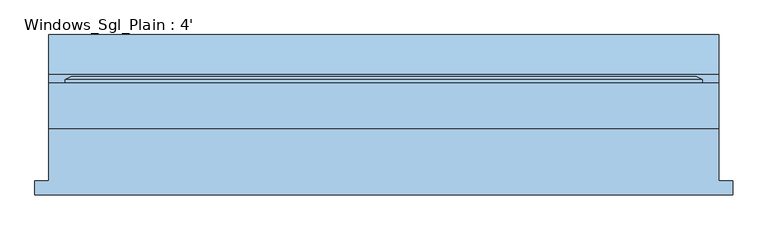
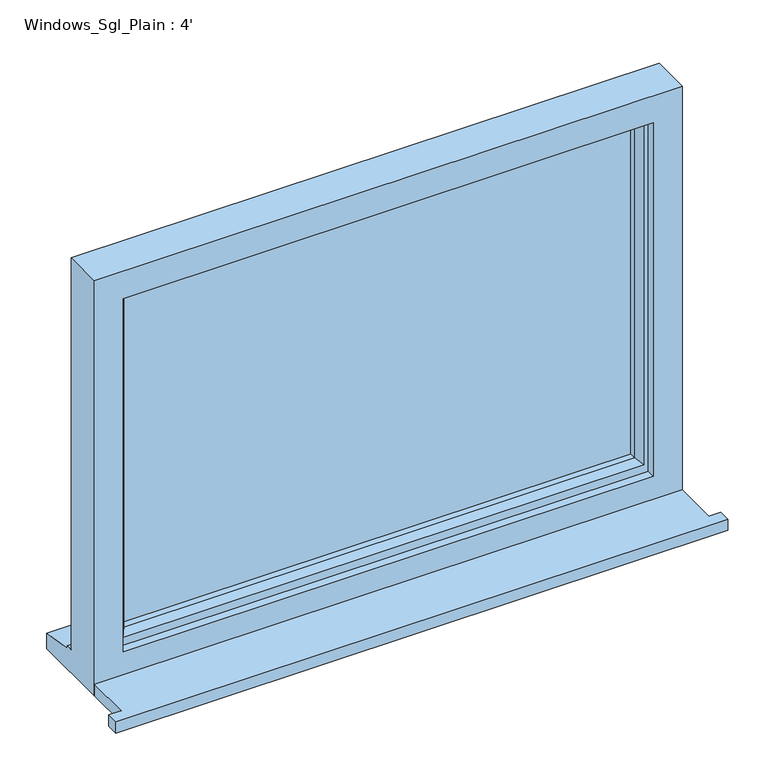
"""IFC4 building model written with IfcOpenShell, lengths in millimetres: window geometry, Windows_Sgl_Plain : 4'."""

from ifc_helpers import new_model, si_unit, frame, origin, place, context, project, spatial, polyline, outline, extrude, faceted_brep, source, transform, mapped, element, save


def windows_sgl_plain_4_aaf4c78a(model_context):
    return source(origin(), model_context, "Body", "SolidModel", [
        extrude(outline(polyline([(-634.6, -130.8434322), (-634.6, -105.8434322), (-609.6, -105.8434322), (-609.6, -10.2434322), (609.6, -10.2434322), (609.6, -105.8434322), (634.6, -105.8434322), (634.6, -130.8434322), (-634.6, -130.8434322)])), frame((0.0, 0.0, 1200.0), z_axis=(0.0, 0.0, 1.0), x_axis=(1.0, 0.0, 0.0)), (0.0, 0.0, 1.0), 25.0),
        faceted_brep([(-609.6, -10.2434322, 1200.0), (609.6, -10.2434322, 1200.0), (609.6, -10.2434322, 2110.0), (-609.6, -10.2434322, 2110.0), (-549.6, -10.2434322, 2050.0), (549.6, -10.2434322, 2050.0), (549.6, -10.2434322, 1275.0), (-549.6, -10.2434322, 1275.0), (-609.6, 72.7565678, 2110.0), (-609.6, 72.7565678, 1251.0), (-609.6, 87.7565678, 1249.68767), (-609.6, 87.7565678, 1244.7449676), (-609.6, 160.2565678, 1233.8088847), (-609.6, 160.2565678, 1200.0), (609.6, 72.7565678, 2110.0), (609.6, 72.7565678, 1251.0), (-569.6, 72.7565678, 2070.0), (-569.6, 72.7565678, 1263.0), (569.6, 72.7565678, 1263.0), (569.6, 72.7565678, 2070.0), (-569.6, 7.7565678, 2070.0), (-569.6, 7.7565678, 1263.0), (569.6, 7.7565678, 2070.0), (569.6, 7.7565678, 1263.0), (-549.6, 7.7565678, 2050.0), (-549.6, 7.7565678, 1275.0), (549.6, 7.7565678, 1275.0), (549.6, 7.7565678, 2050.0), (609.6, 160.2565678, 1200.0), (609.6, 160.2565678, 1233.8088847), (609.6, 87.7565678, 1244.7449676), (609.6, 87.7565678, 1249.68767)], [[[0, 1, 2, 3], [4, 5, 6, 7]], [[0, 3, 8, 9, 10, 11, 12, 13]], [[9, 8, 14, 15], [16, 17, 18, 19]], [[17, 16, 20, 21]], [[20, 22, 23, 21], [24, 25, 26, 27]], [[24, 4, 7, 25]], [[3, 2, 14, 8]], [[16, 19, 22, 20]], [[5, 4, 24, 27]], [[15, 14, 2, 1, 28, 29, 30, 31]], [[19, 18, 23, 22]], [[5, 27, 26, 6]], [[28, 1, 0, 13]], [[29, 28, 13, 12]], [[30, 29, 12, 11]], [[31, 30, 11, 10]], [[15, 31, 10, 9]], [[21, 23, 18, 17]], [[7, 6, 26, 25]]]),
        extrude(outline(polyline([(539.6, 36.7565678), (-539.6, 36.7565678), (-539.6, 60.7565678), (539.6, 60.7565678), (539.6, 36.7565678)])), frame((0.0, 0.0, 1293.0), z_axis=(0.0, 0.0, 1.0), x_axis=(1.0, 0.0, 0.0)), (0.0, 0.0, 1.0), 747.0),
        faceted_brep([(-579.6, 72.7565678, 2080.0), (-579.6, 78.5300705, 2080.0), (-579.6, 78.5300705, 1253.0), (-579.6, 72.7565678, 1253.0), (-569.6, 7.7565678, 2070.0), (-569.6, 72.7565678, 2070.0), (-569.6, 72.7565678, 1263.0), (-569.6, 7.7565678, 1263.0), (-529.6, 22.2494677, 2030.0), (-539.7480377, 7.7565678, 2040.1480377), (-539.7480377, 7.7565678, 1292.8519623), (-529.6, 22.2494677, 1303.0), (-529.6, 36.7565678, 2030.0), (-529.6, 36.7565678, 1303.0), (-539.6, 60.7565678, 2040.0), (-539.6, 36.7565678, 2040.0), (-539.6, 36.7565678, 1293.0), (-539.6, 60.7565678, 1293.0), (-529.6, 78.5300705, 2030.0), (-529.6, 60.7565678, 2030.0), (-529.6, 60.7565678, 1303.0), (-529.6, 78.5300705, 1303.0), (-547.0457548, 84.3035732, 2047.4457548), (-547.0457548, 84.3035732, 1285.5542452), (-568.8153903, 84.3035732, 2069.2153903), (-568.8153903, 84.3035732, 1263.7846097), (579.6, 78.5300705, 1253.0), (579.6, 72.7565678, 1253.0), (569.6, 72.7565678, 1263.0), (569.6, 7.7565678, 1263.0), (539.7480377, 7.7565678, 1292.8519623), (529.6, 22.2494677, 1303.0), (529.6, 36.7565678, 1303.0), (539.6, 36.7565678, 1293.0), (539.6, 60.7565678, 1293.0), (529.6, 60.7565678, 1303.0), (529.6, 78.5300705, 1303.0), (547.0457548, 84.3035732, 1285.5542452), (568.8153903, 84.3035732, 1263.7846097), (579.6, 78.5300705, 2080.0), (579.6, 72.7565678, 2080.0), (569.6, 72.7565678, 2070.0), (569.6, 7.7565678, 2070.0), (539.7480377, 7.7565678, 2040.1480377), (529.6, 22.2494677, 2030.0), (529.6, 36.7565678, 2030.0), (539.6, 36.7565678, 2040.0), (539.6, 60.7565678, 2040.0), (529.6, 60.7565678, 2030.0), (529.6, 78.5300705, 2030.0), (547.0457548, 84.3035732, 2047.4457548), (568.8153903, 84.3035732, 2069.2153903)], [[[0, 1, 2, 3]], [[4, 5, 6, 7]], [[8, 9, 10, 11]], [[12, 8, 11, 13]], [[14, 15, 16, 17]], [[18, 19, 20, 21]], [[22, 18, 21, 23]], [[1, 24, 25, 2]], [[3, 2, 26, 27]], [[7, 6, 28, 29]], [[11, 10, 30, 31]], [[13, 11, 31, 32]], [[17, 16, 33, 34]], [[21, 20, 35, 36]], [[23, 21, 36, 37]], [[2, 25, 38, 26]], [[27, 26, 39, 40]], [[29, 28, 41, 42]], [[31, 30, 43, 44]], [[32, 31, 44, 45]], [[34, 33, 46, 47]], [[36, 35, 48, 49]], [[37, 36, 49, 50]], [[26, 38, 51, 39]], [[40, 39, 1, 0]], [[3, 27, 40, 0], [5, 41, 28, 6]], [[42, 41, 5, 4]], [[7, 29, 42, 4], [9, 43, 30, 10]], [[44, 43, 9, 8]], [[45, 44, 8, 12]], [[15, 46, 33, 16], [13, 32, 45, 12]], [[47, 46, 15, 14]], [[17, 34, 47, 14], [19, 48, 35, 20]], [[49, 48, 19, 18]], [[50, 49, 18, 22]], [[24, 51, 38, 25], [23, 37, 50, 22]], [[39, 51, 24, 1]]]),
    ])


if __name__ == "__main__":
    model = new_model("IFC4")
    model_context = context("Model", 3, world=origin())
    ifc_project = project(units=[si_unit("LENGTHUNIT", "METRE", prefix="MILLI")], contexts=[model_context])
    site = spatial("IfcSite", under=ifc_project)
    building = spatial("IfcBuilding", under=site)
    placement = place(None, origin())
    windows_sgl_plain_4_shape = windows_sgl_plain_4_aaf4c78a(model_context)
    element("IfcWindow", 1, ObjectType="Windows_Sgl_Plain : 4'", at=placement, inside=building, context=model_context, shape_type="MappedRepresentation", body=[
        mapped(windows_sgl_plain_4_shape, transform((0.0, 0.0, 0.0), x_axis=(1.0, 0.0, 0.0), y_axis=(0.0, 1.0, 0.0), z_axis=(0.0, 0.0, 1.0))),
    ])
    save(model, "model.ifc")

# Revit data of these elements
# Type "Windows_Sgl_Plain : 4'"
#   Type Mark = "65"
#   Operation = "SinglePanel"
#   Construction Type Id = "SGL"
#   Manufacturer = "Revit"
#   Keynote = "L10"
#   Analytic Construction = "Large single-glazed windows"
#   Wrap Layers (Ext) from Ext = 0' - 4.03543"
#   Wrap Layers (Int) from Ext = 0' - 6.98819"
#   Window Board Projection = 0' - 0.98425"
#   Window Board Extension = 0' - 0.98425"
#   Visual Light Transmittance = 0.9
#   Solar Heat Gain Coefficient = 0.86
#   Rough Width = 4' - 0"
#   Rough Height = 2' - 11.82677"
#   Height = 2' - 11.82677"
#   Width = 4' - 0"
#   Heat Transfer Coefficient (U) = 5.5617 W/(m²·K)
#   Glazing Thickness = 0' - 0.94488"
#   FrameOffset - External = 0' - 1.9685"
#   Frame Depth = 0' - 2.55906"
#   Default Head Height = 6' - 11.07087"
#   Cill Depth = 0' - 3.44488"
#   Cavity Closer Width = 0' - 1.9685"
#   Cavity Closer Offset from Ext = 0' - 4.03543"
#   Cavity Closer Depth = 0' - 3.34646"
#   Vis - Cavity Closers = yes
#   Define Thermal Properties by = 1
#   Material Trim = Window Frame
#   Material Glass = Glass
#   Material Frame = Window Frame
#   Wall Closure = (empty or 0)
# Element 1 (IfcWindow, "Windows_Sgl_Plain : 4'")
#   Materials on its faces: "Window Frame", "Glass"
# Materials
#   "Window Frame": colour RGB 249 249 249, transparency 0, Keynote = "L10", Cost = 0
#   "Glass": class "Glass", colour RGB 0 128 192, transparency 0.9, Description = "Soda Lime Glass", Cost = 0
